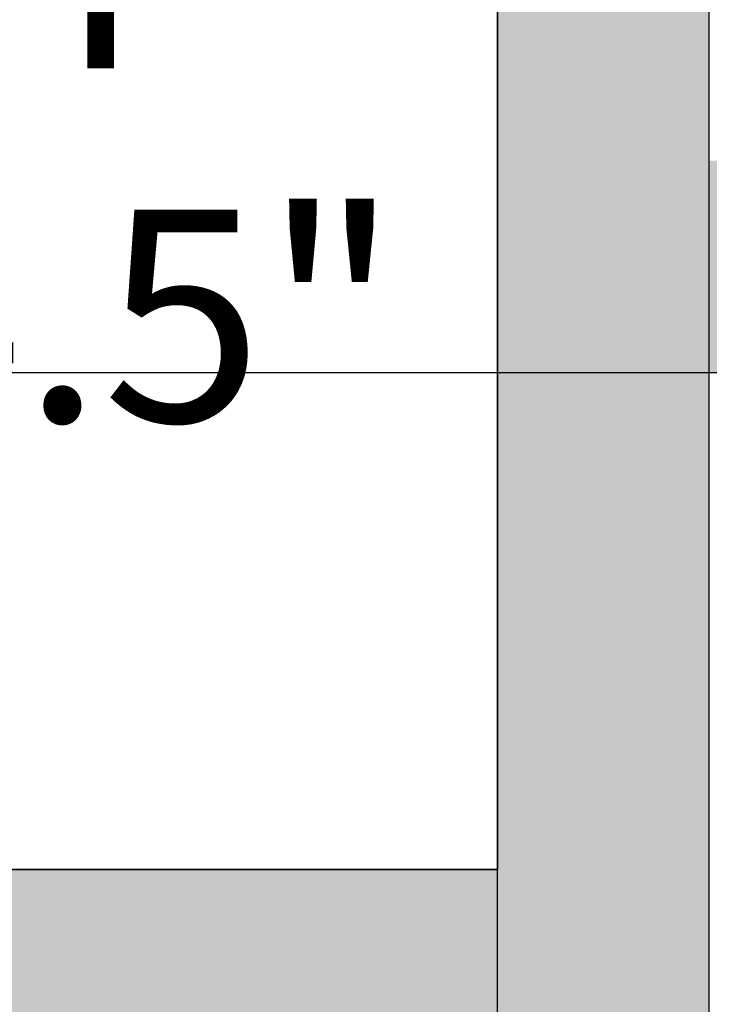
# Model space of a CAD drawing. Units: inches. Extents: x 2696 to 3240, y 1564 to 2310.
# Tile 61 of 76: x 2936 to 2966, y 2180 to 2222. Entities that reach past the tile are written whole.
import ezdxf

# ---------------------------------------------------------------- set-up
doc = ezdxf.new("R2010")
doc.units = ezdxf.units.IN
for name, color, linetype, lineweight in [('A-ANNO-DIMS', 3, 'Continuous', 18), ('A-AREA-IDEN', 7, 'Continuous', 18), ('A-WALL', 7, 'Continuous', 35), ('A-WALL-PATT', 9, 'Continuous', 13)]:
    doc.layers.add(name, color=color, linetype=linetype, lineweight=lineweight)
doc.styles.add('TIMES NEW', font='times.ttf')
doc.styles.add('YQ_DIM', font='SUPEROS.SHX', dxfattribs={"width": 0.8, "bigfont": 'HZDX.SHX'})
doc.dimstyles.new('Siddhuu', dxfattribs={"dimtxt": 6, "dimasz": 2.5, "dimexe": 1.25, "dimexo": 0.625, "dimtad": 1, "dimdec": 1, "dimlunit": 4, "dimtxsty": 'TIMES NEW', "dimcen": 2.5, "dimclrd": 256, "dimclre": 1, "dimclrt": 7, "dimadec": 0, "dimazin": 0, "dimtfac": 1, "dimtdec": 1, "dimtmove": 0, "dimatfit": 3, "dimfxl": 1, "dimtolj": 1, "dimlwd": -1, "dimarcsym": 0})

# ---------------------------------------------------------------- blocks, each defined once
blk = doc.blocks.new('*D59')
at = {"layer": 'A-ANNO-DIMS', "color": 1, "lineweight": -2, "transparency": 16777216}
for p, q in [((2884.709, 1740.826), (2884.709, 2298.451)), ((2956.709, 1740.826), (2956.709, 2298.451))]:
    blk.add_line(p, q, dxfattribs=at)
at = {"layer": 'A-ANNO-DIMS', "transparency": 16777216}
blk.add_line((2887.209, 2297.201), (2954.209, 2297.201), dxfattribs=at)
for points in [[(2887.209, 2297.618), (2887.209, 2296.784), (2884.709, 2297.201)], [(2954.209, 2297.618), (2954.209, 2296.784), (2956.709, 2297.201)]]:
    blk.add_solid(points, dxfattribs=at)
at = {"layer": 'Defpoints', "color": 0, "transparency": 16777216}
for p in [(2956.709, 2297.201), (2884.709, 1740.201), (2956.709, 1740.201)]:
    blk.add_point(p, dxfattribs=at)
at = {"layer": 'A-ANNO-DIMS', "color": 7, "transparency": 16777216, "insert": (2920.709, 2300.878), "char_height": 6, "attachment_point": 5, "style": 'TIMES NEW'}
blk.add_mtext('\\A1;6\'-0"', dxfattribs=at)
blk = doc.blocks.new('*D61')
at = {"layer": 'A-ANNO-DIMS', "color": 1, "lineweight": -2, "transparency": 16777216}
for p, q in [((2965.709, 2141.326), (2965.709, 2298.451)), ((3044.302, 2141.326), (3044.302, 2298.451))]:
    blk.add_line(p, q, dxfattribs=at)
at = {"layer": 'A-ANNO-DIMS', "transparency": 16777216}
blk.add_line((2968.209, 2297.201), (3041.802, 2297.201), dxfattribs=at)
for points in [[(2968.209, 2297.618), (2968.209, 2296.784), (2965.709, 2297.201)], [(3041.802, 2297.618), (3041.802, 2296.784), (3044.302, 2297.201)]]:
    blk.add_solid(points, dxfattribs=at)
at = {"layer": 'Defpoints', "color": 0, "transparency": 16777216}
for p in [(3044.302, 2297.201), (2965.709, 2140.701), (3044.302, 2140.701)]:
    blk.add_point(p, dxfattribs=at)
at = {"layer": 'A-ANNO-DIMS', "color": 7, "transparency": 16777216, "insert": (3005.005, 2300.962), "char_height": 6, "attachment_point": 5, "style": 'TIMES NEW'}
blk.add_mtext('\\A1;6\'-6 1/2"', dxfattribs=at)
blk = doc.blocks.new('*D63')
at = {"layer": 'A-ANNO-DIMS', "color": 1, "lineweight": -2, "transparency": 16777216}
for p, q in [((2965.709, 1989.826), (2965.709, 2298.451)), ((3069.209, 1989.826), (3069.209, 2298.451))]:
    blk.add_line(p, q, dxfattribs=at)
at = {"layer": 'A-ANNO-DIMS', "transparency": 16777216}
blk.add_line((2968.209, 2297.201), (3066.709, 2297.201), dxfattribs=at)
for points in [[(2968.209, 2297.618), (2968.209, 2296.784), (2965.709, 2297.201)], [(3066.709, 2297.618), (3066.709, 2296.784), (3069.209, 2297.201)]]:
    blk.add_solid(points, dxfattribs=at)
at = {"layer": 'Defpoints', "color": 0, "transparency": 16777216}
for p in [(3069.209, 2297.201), (2965.709, 1989.201), (3069.209, 1989.201)]:
    blk.add_point(p, dxfattribs=at)
at = {"layer": 'A-ANNO-DIMS', "color": 7, "transparency": 16777216, "insert": (3017.459, 2300.962), "char_height": 6, "attachment_point": 5, "style": 'TIMES NEW'}
blk.add_mtext('\\A1;8\'-7 1/2"', dxfattribs=at)
blk = doc.blocks.new('*D64')
at = {"layer": 'A-ANNO-DIMS', "color": 1, "lineweight": -2, "transparency": 16777216}
for p, q in [((3073.084, 2206.701), (2709.361, 2206.701)), ((3068.584, 1989.201), (2709.361, 1989.201))]:
    blk.add_line(p, q, dxfattribs=at)
at = {"layer": 'A-ANNO-DIMS', "transparency": 16777216}
blk.add_line((2710.611, 1991.701), (2710.611, 2204.201), dxfattribs=at)
for points in [[(2710.195, 2204.201), (2711.028, 2204.201), (2710.611, 2206.701)], [(2710.195, 1991.701), (2711.028, 1991.701), (2710.611, 1989.201)]]:
    blk.add_solid(points, dxfattribs=at)
at = {"layer": 'Defpoints', "color": 0, "transparency": 16777216}
for p in [(2710.611, 2206.701), (3073.709, 2206.701), (3069.209, 1989.201)]:
    blk.add_point(p, dxfattribs=at)
at = {"layer": 'A-ANNO-DIMS', "color": 7, "transparency": 16777216, "insert": (2706.85, 2097.951), "char_height": 6, "attachment_point": 5, "rotation": 90, "style": 'TIMES NEW'}
blk.add_mtext('\\A1;18\'-1 1/2"', dxfattribs=at)

msp = doc.modelspace()

# ---------------------------------------------------------------- hatches: boundary and pattern name
at = {"layer": 'A-WALL-PATT', "transparency": 33554556}
h = msp.add_hatch(color=256, dxfattribs=at)
h.dxf.hatch_style = 1
h.paths.add_polyline_path([(2879.111, 2253.201), (2905.91, 2253.201), (2905.91, 2262.201), (2841.889, 2262.201), (2841.889, 2253.201), (2870.111, 2253.201), (2870.111, 2176.601), (2965.709, 2176.601), (2965.709, 2206.701), (2973.583, 2206.701), (2973.583, 2215.701), (2965.709, 2215.701), (2965.709, 2262.201), (2929.91, 2262.201), (2929.91, 2253.201), (2956.709, 2253.201), (2956.709, 2185.601), (2879.111, 2185.601)])
h.paths.add_polyline_path([(2782.834, 2262.201), (2745.611, 2262.201), (2745.611, 2228.729), (2754.611, 2228.729), (2754.611, 2253.201), (2782.834, 2253.201)])
h.paths.add_polyline_path([(2754.611, 2136.201), (2965.709, 2136.201), (2965.709, 2145.201), (2879.111, 2145.201), (2879.111, 2147.074), (2877.34, 2147.074), (2870.111, 2147.074), (2870.111, 2145.201), (2754.611, 2145.201), (2754.611, 2169.674), (2745.611, 2169.674), (2745.611, 2000.201), (2754.611, 2000.201), (2754.611, 2019.201), (2849.083, 2019.201), (2849.083, 2023.701), (2841.209, 2023.701), (2841.209, 2051.827), (2836.709, 2051.827), (2836.709, 2023.701), (2754.611, 2023.701), (2754.611, 2091.201), (2836.709, 2091.201), (2836.709, 2087.827), (2841.209, 2087.827), (2841.209, 2095.701), (2754.611, 2095.701)])
h.paths.add_polyline_path([(2965.709, 2136.201), (2956.709, 2136.201), (2956.709, 2023.701), (2885.083, 2023.701), (2885.083, 2019.201), (2956.709, 2019.201), (2956.709, 1950.575), (2965.709, 1950.575), (2965.709, 1980.201), (2973.583, 1980.201), (2973.583, 1989.201), (2965.709, 1989.201)])
h.paths.add_polyline_path([(2754.611, 1906.701), (2880.209, 1906.701), (2884.709, 1906.701), (2956.709, 1906.701), (2956.709, 1792.701), (2944.709, 1792.701), (2944.709, 1783.701), (2956.709, 1783.701), (2956.709, 1740.201), (2884.709, 1740.201), (2884.709, 1783.701), (2896.709, 1783.701), (2896.709, 1792.701), (2884.709, 1792.701), (2884.709, 1846.701), (2880.209, 1846.701), (2880.209, 1740.201), (2754.611, 1740.201), (2754.611, 1777.201), (2745.611, 1777.201), (2745.611, 1692.701), (2754.611, 1692.701), (2754.611, 1731.201), (2956.709, 1731.201), (2956.709, 1723.327), (2965.709, 1723.327), (2965.709, 1884.201), (2973.583, 1884.201), (2973.583, 1893.201), (2965.709, 1893.201), (2965.709, 1914.575), (2956.709, 1914.575), (2956.709, 1911.201), (2754.611, 1911.201), (2754.611, 1930.201), (2745.611, 1930.201), (2745.611, 1817.201), (2754.611, 1817.201), (2754.611, 1854.201), (2826.611, 1854.201), (2826.611, 1868.827), (2822.111, 1868.827), (2822.111, 1858.701), (2754.611, 1858.701)])
h.paths.add_polyline_path([(2965.709, 1656.201), (3008.237, 1656.201), (3008.237, 1665.201), (2965.709, 1665.201), (2965.709, 1693.327), (2956.709, 1693.327), (2956.709, 1686.201), (2934.583, 1686.201), (2934.583, 1681.701), (2956.709, 1681.701), (2956.709, 1614.201), (2896.709, 1614.201), (2896.709, 1681.701), (2904.583, 1681.701), (2904.583, 1686.201), (2892.209, 1686.201), (2892.209, 1614.201), (2858.41, 1614.201), (2858.41, 1605.201), (2965.709, 1605.201)])
h.paths.add_polyline_path([(2788.41, 1614.201), (2754.611, 1614.201), (2754.611, 1652.701), (2745.611, 1652.701), (2745.611, 1605.201), (2788.41, 1605.201)])
h.paths.add_polyline_path([(3199.611, 1633.048), (3190.611, 1633.048), (3190.611, 1614.201), (3082.611, 1614.201), (3082.611, 1665.201), (3070.237, 1665.201), (3070.237, 1656.201), (3078.111, 1656.201), (3078.111, 1605.201), (3199.611, 1605.201)])
h.paths.add_polyline_path([(3199.611, 1702.048), (3190.611, 1702.048), (3190.611, 1699.701), (3106.611, 1699.701), (3106.611, 1747.701), (3190.611, 1747.701), (3190.611, 1752.201), (3082.611, 1752.201), (3082.611, 1760.075), (3078.111, 1760.075), (3078.111, 1747.701), (3102.111, 1747.701), (3102.111, 1699.701), (3078.111, 1699.701), (3078.111, 1695.201), (3190.611, 1695.201), (3190.611, 1676.355), (3199.611, 1676.355)])
h.paths.add_polyline_path([(3199.611, 1783.201), (3190.611, 1783.201), (3190.611, 1745.355), (3199.611, 1745.355)])
h.paths.add_polyline_path([(3082.611, 1884.201), (3190.611, 1884.201), (3190.611, 1853.201), (3199.611, 1853.201), (3199.611, 1901.701), (3190.611, 1901.701), (3190.611, 1893.201), (3005.583, 1893.201), (3005.583, 1891.281), (3005.583, 1884.201), (3078.111, 1884.201), (3078.111, 1792.075), (3082.611, 1792.075)])
h.paths.add_polyline_path([(3199.611, 1994.701), (3190.611, 1994.701), (3190.611, 1989.201), (3073.709, 1989.201), (3073.709, 2034.201), (3069.209, 2034.201), (3069.209, 1989.201), (3005.583, 1989.201), (3005.583, 1980.201), (3190.611, 1980.201), (3190.611, 1971.701), (3199.611, 1971.701)])
h.paths.add_polyline_path([(3199.611, 2155.201), (3190.611, 2155.201), (3190.611, 2064.701), (3199.611, 2064.701)])
h.paths.add_polyline_path([(3190.611, 2074.701), (3106.611, 2074.701), (3106.611, 2122.701), (3190.611, 2122.701), (3190.611, 2127.201), (3082.709, 2127.201), (3082.709, 2135.075), (3073.709, 2135.075), (3073.709, 2122.701), (3102.111, 2122.701), (3102.111, 2074.701), (3069.209, 2074.701), (3069.209, 2070.201), (3190.611, 2070.201)])
h.paths.add_polyline_path([(3082.709, 2253.201), (3190.611, 2253.201), (3190.611, 2225.201), (3199.611, 2225.201), (3199.611, 2262.201), (3073.709, 2262.201), (3073.709, 2215.701), (3035.583, 2215.701), (3035.583, 2206.701), (3073.709, 2206.701), (3073.709, 2171.075), (3082.709, 2171.075)])

# ---------------------------------------------------------------- linework, layer by layer
at = {"layer": 'A-WALL'}
for p, q in [((2956.709, 2185.601), (2956.709, 2253.201)), ((2879.111, 2185.601), (2956.709, 2185.601))]:
    msp.add_line(p, q, dxfattribs=at)

# ---------------------------------------------------------------- texts
at = {"layer": 'A-AREA-IDEN', "insert": (2902.228, 2228.623), "char_height": 9, "attachment_point": 1, "style": 'YQ_DIM'}
msp.add_mtext_dynamic_manual_height_columns('TOILET\\P5\'X5\'4.5"', width=48.00324, gutter_width=12.5, heights=[0], dxfattribs=at)

# ---------------------------------------------------------------- dimensions: what is measured, and where the dimension line sits
at = {"layer": 'A-ANNO-DIMS'}
for base, p1, p2, picture, middle in [((3044.302, 2297.201), (2965.709, 2140.701), (3044.302, 2140.701), '*D61', (3005.005, 2300.962)), ((3069.209, 2297.201), (2965.709, 1989.201), (3069.209, 1989.201), '*D63', (3017.459, 2300.962)), ((2956.709, 2297.201), (2884.709, 1740.201), (2956.709, 1740.201), '*D59', (2920.709, 2300.878))]:
    dim = msp.add_linear_dim(base=base, p1=p1, p2=p2, dimstyle='Siddhuu', override={"dimdec": 1, "dimlfac": 1, "dimrnd": 0, "dimzin": 1, "dimdsep": 46, "dimlunit": 4, "dimfrac": 2}, dxfattribs=at)
    dim.commit()
    dim.dimension.update_dxf_attribs({"geometry": picture, "text_midpoint": middle})
dim = msp.add_linear_dim(base=(2710.611, 2206.701), p1=(3069.209, 1989.201), p2=(3073.709, 2206.701), angle=90, dimstyle='Siddhuu', override={"dimdec": 1, "dimlfac": 1, "dimrnd": 0, "dimzin": 1, "dimdsep": 46, "dimlunit": 4, "dimfrac": 2}, dxfattribs=at)
dim.commit()
dim.dimension.update_dxf_attribs({"geometry": '*D64', "text_midpoint": (2706.85, 2097.951)})

doc.saveas('drawing.dxf')
